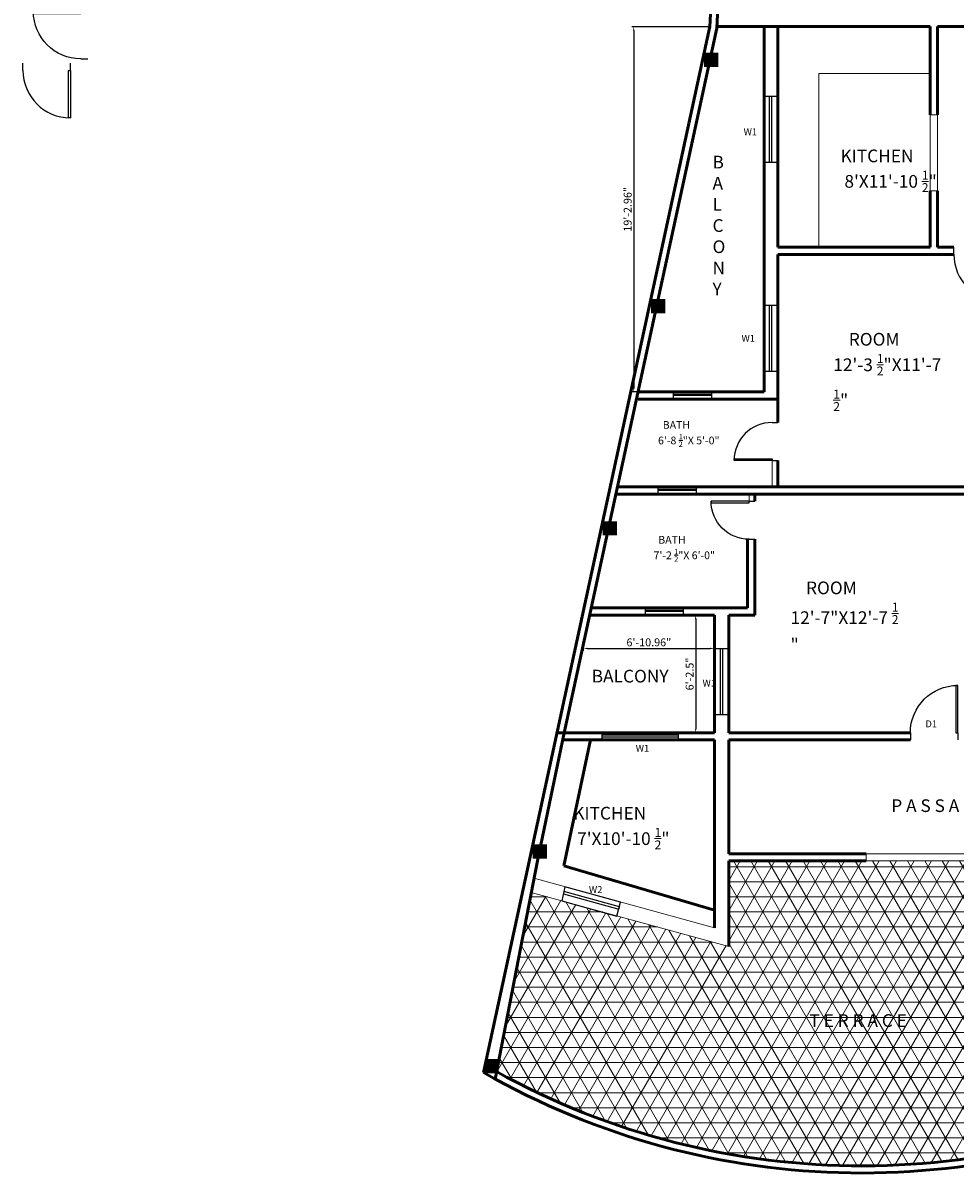
# Model space of a CAD drawing. Units: inches. Extents: x -2733 to 3435, y -338 to 1843.
# Tile 5 of 7: x 643 to 1232, y 349 to 1076. Entities that reach past the tile are written whole.
import ezdxf

# ---------------------------------------------------------------- set-up
doc = ezdxf.new("R2010")
doc.units = ezdxf.units.IN
doc.header["$PDMODE"] = 34
for name, color, linetype, lineweight in [('A-ANNO-DIMS', 2, 'Continuous', 18), ('A-ANNO-TEXT', 7, 'Continuous', 18), ('A-AREA-IDEN', 3, 'Continuous', 18), ('A-COLS', 1, 'Continuous', 35), ('A-DOOR', 1, 'Continuous', 25), ('A-FLOR-FIXT', 8, 'Continuous', 18), ('A-FLOR-PATT', 9, 'Continuous', 13), ('A-GLAZ', 4, 'Continuous', 25), ('A-WALL', 7, 'Continuous', 50)]:
    doc.layers.add(name, color=color, linetype=linetype, lineweight=lineweight)
doc.styles.get("Standard").update_dxf_attribs({"font": 'arial.ttf'})
doc.styles.add('YQ_DIM', font='SUPEROS.SHX', dxfattribs={"width": 0.8, "bigfont": 'HZDX.SHX'})
doc.dimstyles.new('ISO-25', dxfattribs={"dimtxt": 5, "dimasz": 2.5, "dimexe": 1.25, "dimexo": 0.625, "dimtad": 1, "dimlunit": 3, "dimtxsty": 'Standard', "dimcen": 2.5, "dimadec": 0, "dimazin": 0, "dimtfac": 1, "dimtmove": 0, "dimatfit": 3, "dimfxl": 1, "dimarcsym": 0})

# ---------------------------------------------------------------- blocks, each defined once
blk = doc.blocks.new('*U21')
for p, q in [((0, 0), (0, -6)), ((40, 0), (40, -6))]:
    blk.add_line(p, q)
blk.add_lwpolyline([(0, 0), (0, 40), (1.75, 40), (1.75, 0)], close=True)
blk.add_arc((0, 0), 40, 0, 90)
blk = doc.blocks.new('*D25')
at = {"layer": 'A-ANNO-DIMS', "color": 0, "lineweight": -2, "ltscale": 0.5, "transparency": 16777216}
for p, q in [((997.27, 682.56), (997.27, 679.72)), ((999.77, 680.97), (1077.73, 680.97)), ((1080.23, 682.56), (1080.23, 679.72))]:
    blk.add_line(p, q, dxfattribs=at)
at = {"layer": 'A-ANNO-DIMS', "color": 0, "lineweight": 20, "ltscale": 0.5, "transparency": 16777216}
for points in [[(999.77, 681.38), (999.77, 680.55), (997.27, 680.97)], [(1077.73, 681.38), (1077.73, 680.55), (1080.23, 680.97)]]:
    blk.add_solid(points, dxfattribs=at)
at = {"layer": 'Defpoints', "color": 0, "lineweight": 20, "ltscale": 0.5, "transparency": 16777216}
for p in [(997.27, 683.19), (1080.23, 683.19), (1080.23, 680.97)]:
    blk.add_point(p, dxfattribs=at)
at = {"layer": 'A-ANNO-DIMS', "color": 0, "ltscale": 0.5, "transparency": 16777216, "insert": (1038.75, 684.14), "char_height": 5, "attachment_point": 5}
blk.add_mtext('6\'-10.96"', dxfattribs=at)
blk = doc.blocks.new('*D26')
at = {"layer": 'A-ANNO-DIMS', "color": 0, "lineweight": -2, "ltscale": 0.5, "transparency": 16777216}
for p, q in [((1068.36, 699.57), (1068.36, 630.07)), ((1068.99, 702.07), (1069.61, 702.07)), ((1068.99, 627.57), (1069.61, 627.57))]:
    blk.add_line(p, q, dxfattribs=at)
at = {"layer": 'A-ANNO-DIMS', "color": 0, "lineweight": 20, "ltscale": 0.5, "transparency": 16777216}
for points in [[(1067.95, 699.57), (1068.78, 699.57), (1068.36, 702.07)], [(1067.95, 630.07), (1068.78, 630.07), (1068.36, 627.57)]]:
    blk.add_solid(points, dxfattribs=at)
at = {"layer": 'Defpoints', "color": 0, "lineweight": 20, "ltscale": 0.5, "transparency": 16777216}
for p in [(1068.36, 702.07), (1068.36, 627.57), (1068.36, 627.57)]:
    blk.add_point(p, dxfattribs=at)
at = {"layer": 'A-ANNO-DIMS', "color": 0, "ltscale": 0.5, "transparency": 16777216, "insert": (1065.18, 664.82), "char_height": 5, "attachment_point": 5, "rotation": 90}
blk.add_mtext('6\'-2.5"', dxfattribs=at)
blk = doc.blocks.new('*D27')
at = {"layer": 'A-ANNO-DIMS', "color": 0, "lineweight": -2, "ltscale": 0.5, "transparency": 16777216}
for p, q in [((1076.61, 1074.03), (1027.93, 1074.03)), ((1029.18, 1071.53), (1029.18, 845.57)), ((1031.26, 843.07), (1027.93, 843.07))]:
    blk.add_line(p, q, dxfattribs=at)
at = {"layer": 'A-ANNO-DIMS', "color": 0, "lineweight": 20, "ltscale": 0.5, "transparency": 16777216}
for points in [[(1028.76, 1071.53), (1029.6, 1071.53), (1029.18, 1074.03)], [(1028.76, 845.57), (1029.6, 845.57), (1029.18, 843.07)]]:
    blk.add_solid(points, dxfattribs=at)
at = {"layer": 'Defpoints', "color": 0, "lineweight": 20, "ltscale": 0.5, "transparency": 16777216}
for p in [(1077.24, 1074.03), (1029.18, 843.07), (1031.89, 843.07)]:
    blk.add_point(p, dxfattribs=at)
at = {"layer": 'A-ANNO-DIMS', "color": 0, "ltscale": 0.5, "transparency": 16777216, "insert": (1026, 958.55), "char_height": 5, "attachment_point": 5, "rotation": 90}
blk.add_mtext('19\'-2.96"', dxfattribs=at)
blk = doc.blocks.new('WIN-1200')
for points in [[(0, 48), (4.5, 48), (4.5, 0), (0, 0)], [(1.29, 48), (2.82, 48), (2.82, 0), (1.29, 0)]]:
    blk.add_lwpolyline(points, close=True)
blk = doc.blocks.new('WIN-1050')
for points in [[(0, 42), (9, 42), (9, 0), (0, 0)], [(3.84, 42), (5.13, 42), (5.13, 0), (3.84, 0)]]:
    blk.add_lwpolyline(points, close=True)
blk = doc.blocks.new('VENT-600')
at = {"ltscale": 0.5}
for points in [[(0, 24), (4.5, 24), (4.5, 0), (0, 0)], [(1.39, 24), (2.25, 24), (2.25, 0), (1.39, 0)]]:
    blk.add_lwpolyline(points, close=True, dxfattribs=at)

msp = doc.modelspace()

# ---------------------------------------------------------------- hatches: boundary and pattern name
at = {"layer": 'A-COLS'}
h = msp.add_hatch(color=256, dxfattribs=at)
h.dxf.hatch_style = 1
h.paths.add_polyline_path([(1082.621, 1057.541), (1073.621, 1057.541), (1073.621, 1048.541), (1082.621, 1048.541)])
h = msp.add_hatch(color=256, dxfattribs=at)
h.dxf.hatch_style = 1
h.paths.add_polyline_path([(1049.191, 901.828), (1040.191, 901.828), (1040.191, 892.828), (1049.191, 892.828)])
h = msp.add_hatch(color=256, dxfattribs=at)
h.dxf.hatch_style = 1
h.paths.add_polyline_path([(1018.563, 761.378), (1009.563, 761.378), (1009.563, 752.378), (1018.563, 752.378)])
h = msp.add_hatch(color=256, dxfattribs=at)
h.dxf.hatch_style = 1
h.paths.add_polyline_path([(974.298, 557.093), (965.298, 557.093), (965.298, 548.093), (974.298, 548.093)])
h = msp.add_hatch(color=256, dxfattribs=at)
h.dxf.hatch_style = 1
h.paths.add_polyline_path([(943.837, 421.367), (934.837, 421.367), (934.837, 412.367), (943.837, 412.367)])
at = {"layer": 'A-FLOR-PATT'}
h = msp.add_hatch(dxfattribs=at)
h.set_pattern_fill('NET3', color=256, scale=3)
h.paths.add_polyline_path([(1395.735, 546.572), (1089.235, 546.572), (1089.235, 492.572), (964.407, 526.719), (942.472, 413.369, 0.252088), (1395.735, 408.558)])

# ---------------------------------------------------------------- linework, layer by layer
at = {"layer": 'A-FLOR-FIXT'}
for p, q in [((1216.735, 1044.439), (1146.18, 1044.439)), ((1146.18, 1044.439), (1146.18, 934.572)), ((1231.674, 934.572), (1231.674, 930.072)), ((1120.235, 799.792), (1116.635, 799.792)), ((1116.635, 799.792), (1116.635, 783.072)), ((1102.116, 773.958), (1102.116, 778.572)), ((1105.832, 773.958), (1102.116, 773.958)), ((1105.832, 749.958), (1101.216, 749.958)), ((1204.117, 627.572), (1204.117, 623.072)), ((1080.235, 504.365), (966.781, 535.4)), ((1089.235, 492.572), (964.407, 526.719))]:
    msp.add_line(p, q, dxfattribs=at)
at = {"layer": 'A-FLOR-FIXT', "ltscale": 0.5}
for p, q in [((1216.735, 1018.331), (1221.235, 1018.331)), ((1216.735, 1018.331), (1216.735, 970.331)), ((1221.235, 1018.331), (1221.235, 970.331)), ((1221.235, 970.331), (1216.735, 970.331)), ((1176.117, 551.072), (1176.117, 546.572)), ((1176.117, 551.072), (1248.117, 551.072)), ((1248.117, 546.572), (1176.117, 546.572))]:
    msp.add_line(p, q, dxfattribs=at)
at = {"layer": 'A-GLAZ', "ltscale": 0.5}
for p, q in [((985.667, 530.234), (983.804, 521.413)), ((984.736, 525.823), (1019.681, 516.132)), ((1020.097, 517.651), (985.051, 527.318)), ((1020.902, 520.595), (985.667, 530.234)), ((983.804, 521.413), (1018.46, 511.668)), ((1018.46, 511.668), (1020.902, 520.595)), ((1019.681, 516.132), (1020.097, 517.651))]:
    msp.add_line(p, q, dxfattribs=at)
at = {"layer": 'A-WALL'}
for p, q in [((1108.735, 1675.072), (1077.236, 1074.032)), ((1113.229, 1674.837), (1081.697, 1073.183)), ((1077.299, 1074.135), (934.155, 412.879)), ((1081.697, 1073.183), (985.235, 627.572)), ((1216.735, 1074.072), (1081.996, 1074.072)), ((1111.735, 1074.072), (1111.735, 843.073)), ((1120.235, 1074.072), (1120.235, 934.572)), ((1216.735, 1074.072), (1216.735, 1018.331)), ((1395.735, 1074.072), (1221.235, 1074.072)), ((1221.235, 1074.072), (1221.235, 1018.331)), ((1216.735, 970.331), (1216.735, 934.572)), ((1221.235, 970.331), (1221.235, 934.572)), ((1216.735, 934.572), (1120.235, 934.572)), ((1231.674, 934.572), (1221.235, 934.572)), ((1120.235, 930.072), (1120.235, 823.792)), ((1231.674, 930.072), (1120.235, 930.072)), ((1111.735, 843.073), (1031.885, 843.075)), ((1120.235, 838.572), (1031.885, 838.575)), ((1120.235, 799.792), (1120.235, 783.072)), ((1089.235, 778.572), (1017.922, 778.572)), ((1395.735, 783.072), (1018.896, 783.072)), ((1395.735, 778.572), (1089.235, 778.572)), ((1105.832, 773.958), (1105.832, 778.572)), ((1101.216, 749.975), (1101.216, 706.572)), ((1105.832, 701.908), (1105.832, 749.958)), ((1101.216, 706.572), (1002.336, 706.572)), ((1080.235, 702.072), (1001.362, 702.072)), ((1080.235, 702.072), (1080.235, 627.572)), ((1089.235, 701.908), (1089.235, 627.572)), ((1089.235, 701.908), (1101.216, 701.908)), ((1101.216, 701.908), (1105.832, 701.908)), ((985.235, 627.572), (968.249, 546.572)), ((1080.235, 627.572), (980.631, 627.572)), ((1204.117, 627.572), (1089.235, 627.572)), ((1080.235, 623.072), (984.291, 623.072)), ((1080.235, 623.072), (1080.235, 504.365)), ((1080.235, 623.072), (1080.235, 551.072)), ((1204.117, 623.072), (1089.235, 623.072)), ((1089.235, 623.072), (1089.235, 551.072)), ((968.249, 546.572), (941.573, 408.727)), ((1080.235, 546.572), (1080.235, 504.365)), ((1176.117, 551.072), (1089.235, 551.072)), ((1089.235, 546.572), (1089.235, 492.572)), ((1176.117, 546.572), (1089.235, 546.572))]:
    msp.add_line(p, q, dxfattribs=at)
at = {"layer": 'A-WALL', "ltscale": 0.5}
for p, q in [((1001.837, 623.072), (985.026, 543.588)), ((985.026, 543.588), (1080.235, 515.391))]:
    msp.add_line(p, q, dxfattribs=at)
at = {"layer": 'A-WALL'}
for radius, start, end in [(478.102, 240.087713, 298.300235), (482.602, 240.258112, 298.012953)]:
    msp.add_arc((1173.571, 831.907), radius, start, end, dxfattribs=at)

# ---------------------------------------------------------------- block references
at = {"layer": 'A-DOOR'}
for p, xscale, yscale, zscale, rotation in [((679.505, 1083.717), -0.75, 0.75, 0.75, 90), ((672.93, 1046.378), 0.75, 0.75, 0.75, 180), ((1261.674, 930.156), 0.75, 0.75, 0.75, 180), ((1116.635, 799.792), 0.6, 0.6, 0.6, 90), ((1102.116, 773.958), -0.6, 0.6, 0.6, 90)]:
    msp.add_blockref('*U21', p, dxfattribs=dict(at, xscale=xscale, yscale=yscale, zscale=zscale, rotation=rotation))
at = {"layer": 'A-DOOR', "xscale": -0.75, "yscale": 0.75, "zscale": 0.75}
msp.add_blockref('*U21', (1234.117, 627.572), dxfattribs=at)
at = {"layer": 'A-GLAZ'}
for p in [(1111.235, 988.18), (1111.235, 855.932), (1080.235, 638.967)]:
    msp.add_blockref('WIN-1050', p, dxfattribs=at)
for name, p, rotation in [('VENT-600', (1054.282, 843.074), 270.0000000000016), ('VENT-600', (1044.634, 783.072), 270.0000000000014), ('VENT-600', (1036.538, 706.572), 270.0000000000001), ('WIN-1200', (1009.249, 627.572), 269.9999999999995)]:
    msp.add_blockref(name, p, dxfattribs=dict(at, rotation=rotation))

# ---------------------------------------------------------------- texts
at = {"layer": 'A-ANNO-TEXT', "ltscale": 0.5, "char_height": 4.35068, "attachment_point": 1, "style": 'YQ_DIM'}
for s, insert in [('{\\f@Arial Unicode MS|b0|i0|c0|p34;W1}', (1098.686, 1009.729)), ('{\\f@Arial Unicode MS|b0|i0|c0|p34;W1}', (1097.359, 879.2)), ('{\\f@Arial Unicode MS|b0|i0|c0|p34;W1}', (1072.7, 661.224)), ('{\\f@Arial Unicode MS|b0|i0|c0|p34;D1}', (1213.656, 635.438)), ('{\\f@Arial Unicode MS|b0|i0|c0|p34;W1}', (1030.47, 619.926)), ('{\\f@Arial Unicode MS|b0|i0|c0|p34;W2}', (1000.854, 530.658))]:
    msp.add_mtext_dynamic_manual_height_columns(s, width=7.90712, gutter_width=21.753, heights=[0], dxfattribs=dict(at, insert=insert))
at = {"layer": 'A-AREA-IDEN', "ltscale": 0.5, "attachment_point": 1, "style": 'YQ_DIM'}
for s, width, gutter_width, heights, insert, char_height in [('\\A1; {\\fMicrosoft YaHei UI|b0|i0|c0|p34;KITCHEN\\P  8\'X11\'-10 \\H0.7x;\\S1/2;\\H1.42857x;"}', 67.57438, 12.5, [43.34], (1157.531, 996.332), 8.02), ('{\\fAcadEref|b0|i0|c0|p2;B\\f@Arial Unicode MS|b1|i1|c0|p34; A\\PL\\PC\\PO\\PN\\PY}', 12.11312, 12.5, [99.959], (1079.01, 992.41), 8.02), ('\\A1;{\\f@Malgun Gothic|b0|i0|c0|p34;    ROOM \\P12\'-3 \\H0.7x;\\S1/2;\\H1.42857x;"X11\'-7 \\H0.7x;\\S1/2;\\H1.42857x;"}', 69.89446, 40.122, [0], (1155.386, 880.406), 8.02448), ('\\A1;{  \\fSegoe UI Black|b0|i0|c0|p34;BATH\\P6\'-8 \\H0.7x;\\S1/2;\\H1.42857x;"X 5\'-0"}', 43.60909, 24.448, [0], (1044.561, 824.687), 4.88966), ('\\A1;{  \\fSegoe UI Black|b0|i0|c0|p34;BATH\\P7\'-2 \\H0.7x;\\S1/2;\\H1.42857x;"X 6\'-0"}', 43.60909, 24.448, [0], (1041.718, 752.071), 4.88966), ('\\A1;{\\f@Malgun Gothic|b0|i0|c0|p34;    ROOM \\P12\'-7\\H1x;"X12\'-7 \\H0.7x;\\S1/2;\\H1.42857x;"}', 69.89446, 40.122, [0], (1128.35, 723.245), 8.02448), ('\\A1;{\\fGabriola|b0|i0|c0|p82;BALCONY}', 67.57438, 12.5, [14.95], (1002.601, 667.434), 8.02), ('\\A1; {\\fMicrosoft YaHei UI|b0|i0|c0|p34;KITCHEN\\P  7\'X10\'-10 \\H0.7x;\\S1/2;\\H1.42857x;"}', 67.57438, 12.5, [43.34], (988.5, 580.798), 8.02), ('{\\f@Arial Unicode MS|b0|i0|c0|p34;T E R R A C E}', 108.12884, 12.5, [1.216], (1140.274, 449.692), 8.02)]:
    msp.add_mtext_dynamic_manual_height_columns(s, width=width, gutter_width=gutter_width, heights=heights, dxfattribs=dict(at, insert=insert, char_height=char_height))
at = {"layer": 'A-AREA-IDEN', "insert": (1231.87, 581.536), "char_height": 8, "attachment_point": 5, "style": 'YQ_DIM'}
msp.add_mtext_dynamic_manual_height_columns("{\\f@MS PGothic|b0|i0|c0|p34;P A S S A G E - 6'}", width=111.08232, gutter_width=12.5, heights=[0], dxfattribs=at)

# ---------------------------------------------------------------- dimensions: what is measured, and where the dimension line sits
at = {"layer": 'A-ANNO-DIMS', "ltscale": 0.5}
for base, p1, p2, picture, middle in [((1029.18, 843.075), (1077.236, 1074.032), (1031.885, 843.075), '*D27', (1026.002, 958.554)), ((1068.362, 627.572), (1068.362, 702.072), (1068.362, 627.572), '*D26', (1065.184, 664.822))]:
    dim = msp.add_linear_dim(base=base, p1=p1, p2=p2, angle=90, dimstyle='ISO-25', override={"dimclrd": 0, "dimclre": 0, "dimclrt": 0}, dxfattribs=at)
    dim.commit()
    dim.dimension.update_dxf_attribs({"geometry": picture, "text_midpoint": middle})
dim = msp.add_linear_dim(base=(1080.235, 680.967), p1=(997.274, 683.188), p2=(1080.235, 683.188), dimstyle='ISO-25', override={"dimclrd": 0, "dimclre": 0, "dimclrt": 0}, dxfattribs=at)
dim.commit()
dim.dimension.update_dxf_attribs({"geometry": '*D25', "text_midpoint": (1038.755, 684.145)})

doc.saveas('drawing.dxf')
